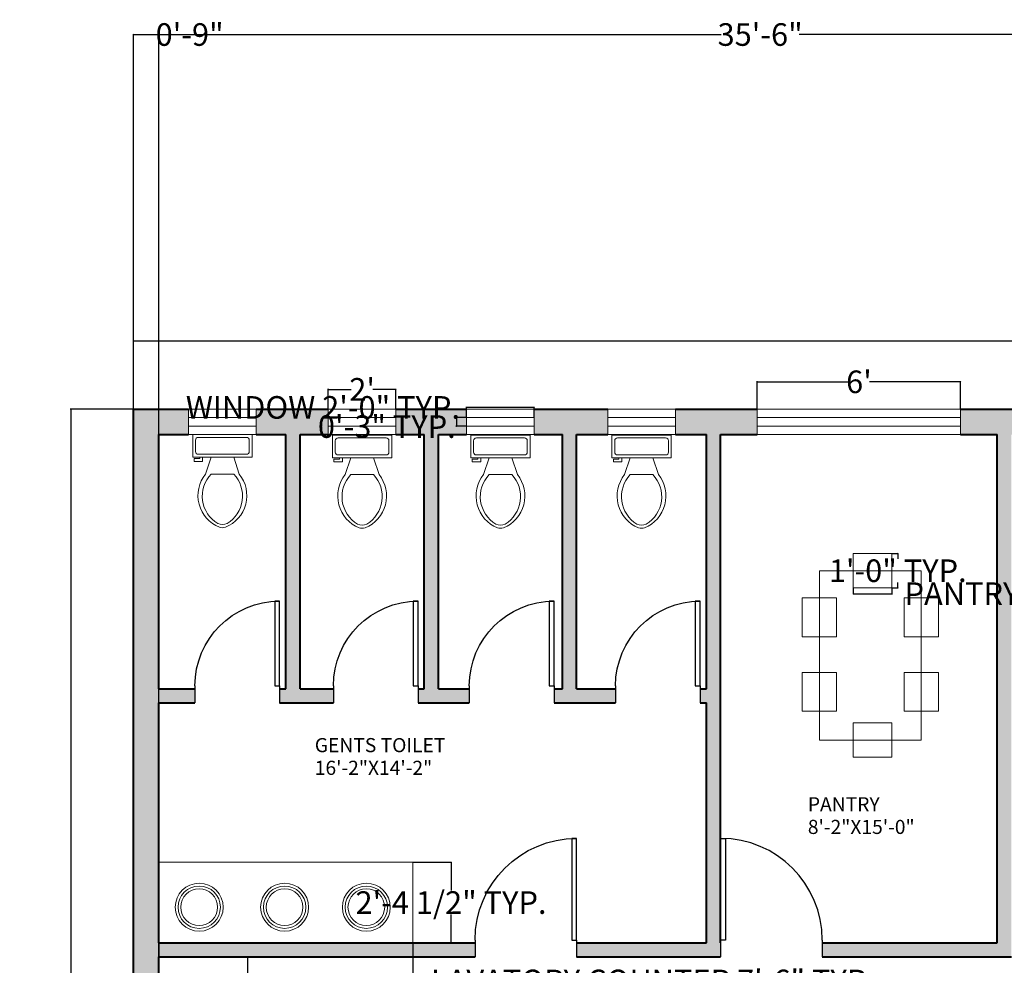
# Model space of a CAD drawing. Units: inches. Extents: x -405 to 940, y 226 to 2032.
# Tile 6 of 10: x -298 to 51, y 1691 to 2026. Entities that reach past the tile are written whole.
import ezdxf

# ---------------------------------------------------------------- set-up
doc = ezdxf.new("R2010")
doc.units = ezdxf.units.IN
doc.header["$MEASUREMENT"] = 0
doc.linetypes.add('ACAD_ISO02W100', pattern=[15, 12, -3])
for name, color, linetype, lineweight in [('A-ANNO-DIMS', 120, 'Continuous', 18), ('A-AREA-IDEN', 32, 'Continuous', 18), ('A-FLOR-FIXT', 175, 'Continuous', 18), ('A-FURN-SEAT', 5, 'Continuous', 18), ('A-GLAZ-HIDN', 1, 'ACAD_ISO02W100', 18), ('A-WALL-PATT', 8, 'Continuous', 13), ('door', 6, 'Continuous', 25), ('tables', 2, 'Continuous', 18), ('wall', 3, 'Continuous', 40), ('window', 1, 'Continuous', 18)]:
    doc.layers.add(name, color=color, linetype=linetype, lineweight=lineweight)
doc.styles.get("Standard").update_dxf_attribs({"font": 'arial.ttf'})
doc.dimstyles.get("Standard").update_dxf_attribs({"dimtxt": 8, "dimasz": 0.18, "dimexe": 0.18, "dimexo": 0.0625, "dimgap": 0.09, "dimtad": 0, "dimtih": 1, "dimtoh": 1, "dimdec": 0, "dimzin": 0, "dimdsep": 46, "dimlunit": 3, "dimtxsty": 'Standard', "dimblk": 'OBLIQUE', "dimcen": 0.09, "dimadec": 0, "dimazin": 0, "dimtfac": 1, "dimtdec": 0, "dimtofl": 0, "dimtmove": 0, "dimatfit": 3, "dimfxl": 1, "dimtolj": 1, "dimtzin": 0, "dimarcsym": 0})

# ---------------------------------------------------------------- blocks, each defined once
blk = doc.blocks.new('*U3')
for p, q in [((0, 0), (0, -6)), ((30, 0), (30, -6))]:
    blk.add_line(p, q)
blk.add_lwpolyline([(0, 0), (0, 30), (1.75, 30), (1.75, 0)], close=True)
blk.add_arc((0, 0), 30, 0, 90)
blk = doc.blocks.new('*U4')
for p, q in [((0, 0), (0, -6)), ((36, 0), (36, -6))]:
    blk.add_line(p, q)
blk.add_lwpolyline([(0, 0), (0, 36), (1.75, 36), (1.75, 0)], close=True)
blk.add_arc((0, 0), 36, 0, 90)
blk = doc.blocks.new('*U6')
for p, q in [((9.5, -6), (9.5, -2)), ((-10, -8.5), (-8, -8.5)), ((-10, -9.5), (-10, -8.5)), ((-7, -9.5), (-10, -9.5)), ((-8, -8.5), (-8, -8)), ((-7, -8), (-7, -9.5)), ((-4, -8), (-6, -14)), ((4, -8), (6, -14)), ((4, -14), (-4, -14))]:
    blk.add_line(p, q)
blk.add_lwpolyline([(10.5, -8), (10.5, 0), (-10.5, 0), (-10.5, -8)], close=True)
for points in [[(-9.5, -2), (-9.5, -6)], [(8.5, -1), (-8.5, -1)], [(-8.5, -7), (8.5, -7)]]:
    blk.add_lwpolyline(points)
for centre, radius, start, end in [((-8.62, -1.88), 0.884, 81.8699, 188.1301), ((8.62, -1.88), 0.884, 351.8699, 98.1301), ((-8.62, -6.12), 0.884, 171.8699, 278.1301), ((8.62, -6.12), 0.884, 261.8699, 8.1301), ((3.52, -21.58), 12.17, 141.4691, 247.9714), ((4.2, -21.82), 11.33, 136.3677, 238.9468), ((-3.52, -21.58), 12.17, 292.0284, 38.5307), ((-4.2, -21.82), 11.33, 301.053, 43.6321), ((0, -27.88), 4, 245.7318, 294.2682), ((0, -29), 4, 254.8605, 285.1395)]:
    blk.add_arc(centre, radius, start, end)
blk = doc.blocks.new('_Oblique')
at = {"color": 0, "linetype": 'ByBlock', "lineweight": -2}
blk.add_line((-0.5, -0.5), (0.5, 0.5), dxfattribs=at)
blk = doc.blocks.new('*D43')
at = {"layer": 'A-ANNO-DIMS', "color": 0, "lineweight": -2, "transparency": 16777216}
for p, q in [((-257.23, 1887.87), (-257.23, 1912.15)), ((-257.23, 1911.97), (265.43, 1911.97)), ((815.77, 1911.97), (293.1, 1911.97)), ((815.77, 1887.87), (815.77, 1912.15))]:
    blk.add_line(p, q, dxfattribs=at)
at = {"layer": 'Defpoints', "color": 0, "transparency": 16777216}
for p in [(815.77, 1911.97), (-257.23, 1887.81), (815.77, 1887.81)]:
    blk.add_point(p, dxfattribs=at)
at = {"layer": 'A-ANNO-DIMS', "color": 0, "lineweight": -2, "transparency": 16777216, "xscale": 0.18, "yscale": 0.18, "zscale": 0.18, "rotation": 180}
blk.add_blockref('_Oblique', (-257.23, 1911.97), dxfattribs=at)
at = {"layer": 'A-ANNO-DIMS', "color": 0, "lineweight": -2, "transparency": 16777216, "xscale": 0.18, "yscale": 0.18, "zscale": 0.18}
blk.add_blockref('_Oblique', (815.77, 1911.97), dxfattribs=at)
at = {"layer": 'A-ANNO-DIMS', "color": 0, "transparency": 16777216, "insert": (279.27, 1911.97), "char_height": 8, "attachment_point": 5}
blk.add_mtext('\\A1;89\'-5"', dxfattribs=at)
blk = doc.blocks.new('*D44')
at = {"layer": 'A-ANNO-DIMS', "color": 0, "lineweight": -2, "transparency": 16777216}
for p, q in [((-257.29, 1887.81), (-279.61, 1887.81)), ((-279.43, 1887.81), (-279.43, 1210.99)), ((-279.43, 525.81), (-279.43, 1202.63)), ((-257.29, 525.81), (-279.61, 525.81))]:
    blk.add_line(p, q, dxfattribs=at)
at = {"layer": 'Defpoints', "color": 0, "transparency": 16777216}
for p in [(-257.23, 1887.81), (-279.43, 525.81), (-257.23, 525.81)]:
    blk.add_point(p, dxfattribs=at)
at = {"layer": 'A-ANNO-DIMS', "color": 0, "lineweight": -2, "transparency": 16777216, "xscale": 0.18, "yscale": 0.18, "zscale": 0.18}
for p, rotation in [((-279.43, 1887.81), 90), ((-279.43, 525.81), 270)]:
    blk.add_blockref('_Oblique', p, dxfattribs=dict(at, rotation=rotation))
at = {"layer": 'A-ANNO-DIMS', "color": 0, "transparency": 16777216, "insert": (-279.43, 1206.81), "char_height": 8, "attachment_point": 5}
blk.add_mtext('\\A1;113\'-6"', dxfattribs=at)
blk = doc.blocks.new('*D59')
at = {"layer": 'A-ANNO-DIMS', "color": 0, "lineweight": -2, "transparency": 16777216}
for p, q in [((-218.67, 1693.81), (-216.61, 1693.81)), ((-216.79, 1693.81), (-216.79, 1655.9)), ((-216.79, 1609.81), (-216.79, 1647.72)), ((-218.67, 1609.81), (-216.61, 1609.81))]:
    blk.add_line(p, q, dxfattribs=at)
at = {"layer": 'Defpoints', "color": 0, "transparency": 16777216}
for p in [(-218.73, 1693.81), (-218.73, 1609.81), (-216.79, 1609.81)]:
    blk.add_point(p, dxfattribs=at)
at = {"layer": 'A-ANNO-DIMS', "color": 0, "lineweight": -2, "transparency": 16777216, "xscale": 0.18, "yscale": 0.18, "zscale": 0.18}
for p, rotation in [((-216.79, 1693.81), 90), ((-216.79, 1609.81), 270)]:
    blk.add_blockref('_Oblique', p, dxfattribs=dict(at, rotation=rotation))
at = {"layer": 'A-ANNO-DIMS', "color": 0, "transparency": 16777216, "insert": (-216.79, 1651.81), "char_height": 8, "attachment_point": 5}
blk.add_mtext("\\A1;7'", dxfattribs=at)
blk = doc.blocks.new('*D61')
at = {"layer": 'A-ANNO-DIMS', "color": 0, "lineweight": -2, "transparency": 16777216}
for p, q in [((-188.23, 1887.87), (-188.23, 1894.99)), ((-188.23, 1894.81), (-180.07, 1894.81)), ((-164.23, 1894.81), (-172.39, 1894.81)), ((-164.23, 1887.87), (-164.23, 1894.99))]:
    blk.add_line(p, q, dxfattribs=at)
at = {"layer": 'Defpoints', "color": 0, "transparency": 16777216}
for p in [(-164.23, 1894.81), (-188.23, 1887.81), (-164.23, 1887.81)]:
    blk.add_point(p, dxfattribs=at)
at = {"layer": 'A-ANNO-DIMS', "color": 0, "lineweight": -2, "transparency": 16777216, "xscale": 0.18, "yscale": 0.18, "zscale": 0.18, "rotation": 180}
blk.add_blockref('_Oblique', (-188.23, 1894.81), dxfattribs=at)
at = {"layer": 'A-ANNO-DIMS', "color": 0, "lineweight": -2, "transparency": 16777216, "xscale": 0.18, "yscale": 0.18, "zscale": 0.18}
blk.add_blockref('_Oblique', (-164.23, 1894.81), dxfattribs=at)
at = {"layer": 'A-ANNO-DIMS', "color": 0, "transparency": 16777216, "insert": (-176.23, 1894.81), "char_height": 8, "attachment_point": 5}
blk.add_mtext("\\A1;2'", dxfattribs=at)
blk = doc.blocks.new('*D62')
at = {"layer": 'A-ANNO-DIMS', "color": 0, "lineweight": -2, "transparency": 16777216}
for p, q in [((-36.23, 1887.87), (-36.23, 1897.66)), ((35.77, 1887.87), (35.77, 1897.66)), ((-36.23, 1897.48), (-4.02, 1897.48)), ((35.77, 1897.48), (3.56, 1897.48))]:
    blk.add_line(p, q, dxfattribs=at)
at = {"layer": 'Defpoints', "color": 0, "transparency": 16777216}
for p in [(35.77, 1897.48), (-36.23, 1887.81), (35.77, 1887.81)]:
    blk.add_point(p, dxfattribs=at)
at = {"layer": 'A-ANNO-DIMS', "color": 0, "lineweight": -2, "transparency": 16777216, "xscale": 0.18, "yscale": 0.18, "zscale": 0.18, "rotation": 180}
blk.add_blockref('_Oblique', (-36.23, 1897.48), dxfattribs=at)
at = {"layer": 'A-ANNO-DIMS', "color": 0, "lineweight": -2, "transparency": 16777216, "xscale": 0.18, "yscale": 0.18, "zscale": 0.18}
blk.add_blockref('_Oblique', (35.77, 1897.48), dxfattribs=at)
at = {"layer": 'A-ANNO-DIMS', "color": 0, "transparency": 16777216, "insert": (-0.23, 1897.48), "char_height": 8, "attachment_point": 5}
blk.add_mtext("\\A1;6'", dxfattribs=at)
blk = doc.blocks.new('LAVATORY-COUNTER-TRIPLE')
for p, q in [((0, 28.51), (89.99, 28.51)), ((89.99, 28.51), (89.99, 0))]:
    blk.add_line(p, q)
for centre, radius in [((14.28, 12.62), 8.5), ((44.55, 12.62), 8.5), ((73.49, 12.62), 8.5), ((14.28, 12.62), 7.5), ((14.28, 12.62), 6.5), ((44.55, 12.62), 7.5), ((44.55, 12.62), 6.5), ((73.49, 12.62), 7.5), ((73.49, 12.62), 6.5)]:
    blk.add_circle(centre, radius)
blk = doc.blocks.new('CHAIR-PANTRY')
blk.add_lwpolyline([(0, 12.15), (13.72, 12.15), (13.72, 0), (0, 0)], close=True)
blk = doc.blocks.new('WIN-PANE-24IN')
for p, q in [((0, 3), (24, 3)), ((0, 0), (24, 0))]:
    blk.add_line(p, q)
blk = doc.blocks.new('WIN-PANE-72IN')
for p, q in [((0, 3), (72, 3)), ((0, 0), (72, 0))]:
    blk.add_line(p, q)
blk = doc.blocks.new('*D85')
at = {"layer": 'A-ANNO-DIMS', "color": 0, "lineweight": -2, "transparency": 16777216}
for p, q in [((-139.23, 1888.41), (-139.41, 1888.41)), ((-139.23, 1884.87), (-139.23, 1888.59)), ((-115.23, 1888.41), (-139.23, 1888.41)), ((-115.23, 1884.87), (-115.23, 1888.59))]:
    blk.add_line(p, q, dxfattribs=at)
at = {"layer": 'Defpoints', "color": 0, "transparency": 16777216}
for p in [(-139.23, 1888.41), (-139.23, 1884.81), (-115.23, 1884.81)]:
    blk.add_point(p, dxfattribs=at)
at = {"layer": 'A-ANNO-DIMS', "color": 0, "lineweight": -2, "transparency": 16777216, "xscale": 0.18, "yscale": 0.18, "zscale": 0.18, "rotation": 180}
blk.add_blockref('_Oblique', (-139.23, 1888.41), dxfattribs=at)
at = {"layer": 'A-ANNO-DIMS', "color": 0, "lineweight": -2, "transparency": 16777216, "xscale": 0.18, "yscale": 0.18, "zscale": 0.18}
blk.add_blockref('_Oblique', (-115.23, 1888.41), dxfattribs=at)
at = {"layer": 'A-ANNO-DIMS', "color": 0, "transparency": 16777216, "insert": (-190.12, 1888.41), "char_height": 8, "attachment_point": 5}
blk.add_mtext('\\A1;WINDOW 2\'-0" TYP.', dxfattribs=at)
blk = doc.blocks.new('*D86')
at = {"layer": 'A-ANNO-DIMS', "color": 0, "lineweight": -2, "transparency": 16777216}
for p, q in [((-139.29, 1884.81), (-143.01, 1884.81)), ((-142.83, 1884.81), (-142.83, 1881.81)), ((-139.29, 1881.81), (-143.01, 1881.81)), ((-142.83, 1881.63), (-143.01, 1881.63)), ((-142.83, 1881.81), (-142.83, 1881.63))]:
    blk.add_line(p, q, dxfattribs=at)
at = {"layer": 'Defpoints', "color": 0, "transparency": 16777216}
for p in [(-139.23, 1884.81), (-142.83, 1881.81), (-139.23, 1881.81)]:
    blk.add_point(p, dxfattribs=at)
at = {"layer": 'A-ANNO-DIMS', "color": 0, "lineweight": -2, "transparency": 16777216, "xscale": 0.18, "yscale": 0.18, "zscale": 0.18}
for p, rotation in [((-142.83, 1884.81), 90), ((-142.83, 1881.81), 270)]:
    blk.add_blockref('_Oblique', p, dxfattribs=dict(at, rotation=rotation))
at = {"layer": 'A-ANNO-DIMS', "color": 0, "transparency": 16777216, "insert": (-167.48, 1881.63), "char_height": 8, "attachment_point": 5}
blk.add_mtext('\\A1;0\'-3" TYP.', dxfattribs=at)
blk = doc.blocks.new('*D91')
at = {"layer": 'A-ANNO-DIMS', "color": 0, "lineweight": -2, "transparency": 16777216}
for p, q in [((-2.26, 1824.45), (-2.26, 1822.27)), ((11.46, 1824.45), (11.46, 1822.27)), ((-2.26, 1822.45), (11.46, 1822.45)), ((11.46, 1822.45), (11.64, 1822.45))]:
    blk.add_line(p, q, dxfattribs=at)
at = {"layer": 'Defpoints', "color": 0, "transparency": 16777216}
for p in [(-2.26, 1824.51), (11.46, 1824.51), (11.46, 1822.45)]:
    blk.add_point(p, dxfattribs=at)
at = {"layer": 'A-ANNO-DIMS', "color": 0, "lineweight": -2, "transparency": 16777216, "xscale": 0.18, "yscale": 0.18, "zscale": 0.18, "rotation": 180}
blk.add_blockref('_Oblique', (-2.26, 1822.45), dxfattribs=at)
at = {"layer": 'A-ANNO-DIMS', "color": 0, "lineweight": -2, "transparency": 16777216, "xscale": 0.18, "yscale": 0.18, "zscale": 0.18}
blk.add_blockref('_Oblique', (11.46, 1822.45), dxfattribs=at)
at = {"layer": 'A-ANNO-DIMS', "color": 0, "transparency": 16777216, "insert": (88.39, 1822.45), "char_height": 8, "attachment_point": 5}
blk.add_mtext('\\A1;PANTRY CHAIR 1\'-1 1/2" TYP.', dxfattribs=at)
blk = doc.blocks.new('*D92')
at = {"layer": 'A-ANNO-DIMS', "color": 0, "lineweight": -2, "transparency": 16777216}
for p, q in [((11.53, 1836.66), (13.7, 1836.66)), ((13.52, 1836.66), (13.52, 1834.76)), ((11.53, 1824.51), (13.7, 1824.51)), ((13.52, 1824.51), (13.52, 1826.41))]:
    blk.add_line(p, q, dxfattribs=at)
at = {"layer": 'Defpoints', "color": 0, "transparency": 16777216}
for p in [(11.46, 1836.66), (13.52, 1836.66), (11.46, 1824.51)]:
    blk.add_point(p, dxfattribs=at)
at = {"layer": 'A-ANNO-DIMS', "color": 0, "lineweight": -2, "transparency": 16777216, "xscale": 0.18, "yscale": 0.18, "zscale": 0.18}
for p, rotation in [((13.52, 1836.66), 90), ((13.52, 1824.51), 270)]:
    blk.add_blockref('_Oblique', p, dxfattribs=dict(at, rotation=rotation))
at = {"layer": 'A-ANNO-DIMS', "color": 0, "transparency": 16777216, "insert": (13.52, 1830.58), "char_height": 8, "attachment_point": 5}
blk.add_mtext('\\A1;1\'-0" TYP.', dxfattribs=at)
blk = doc.blocks.new('*D93')
at = {"layer": 'A-ANNO-DIMS', "color": 0, "lineweight": -2, "transparency": 16777216}
for p, q in [((-248.23, 1698.75), (-248.23, 1685.13)), ((-158.24, 1698.75), (-158.24, 1685.13)), ((-248.23, 1685.31), (-158.24, 1685.31)), ((-158.24, 1685.31), (-158.06, 1685.31))]:
    blk.add_line(p, q, dxfattribs=at)
at = {"layer": 'Defpoints', "color": 0, "transparency": 16777216}
for p in [(-248.23, 1698.81), (-158.24, 1698.81), (-158.24, 1685.31)]:
    blk.add_point(p, dxfattribs=at)
at = {"layer": 'A-ANNO-DIMS', "color": 0, "lineweight": -2, "transparency": 16777216, "xscale": 0.18, "yscale": 0.18, "zscale": 0.18, "rotation": 180}
blk.add_blockref('_Oblique', (-248.23, 1685.31), dxfattribs=at)
at = {"layer": 'A-ANNO-DIMS', "color": 0, "lineweight": -2, "transparency": 16777216, "xscale": 0.18, "yscale": 0.18, "zscale": 0.18}
blk.add_blockref('_Oblique', (-158.24, 1685.31), dxfattribs=at)
at = {"layer": 'A-ANNO-DIMS', "color": 0, "transparency": 16777216, "insert": (-73.22, 1685.31), "char_height": 8, "attachment_point": 5}
blk.add_mtext('\\A1;LAVATORY COUNTER 7\'-6" TYP.', dxfattribs=at)
blk = doc.blocks.new('*D94')
at = {"layer": 'A-ANNO-DIMS', "color": 0, "lineweight": -2, "transparency": 16777216}
for p, q in [((-158.18, 1727.32), (-144.56, 1727.32)), ((-144.74, 1727.32), (-144.74, 1717.29)), ((-144.74, 1698.81), (-144.74, 1708.84)), ((-158.18, 1698.81), (-144.56, 1698.81))]:
    blk.add_line(p, q, dxfattribs=at)
at = {"layer": 'Defpoints', "color": 0, "transparency": 16777216}
for p in [(-158.24, 1727.32), (-144.74, 1727.32), (-158.24, 1698.81)]:
    blk.add_point(p, dxfattribs=at)
at = {"layer": 'A-ANNO-DIMS', "color": 0, "lineweight": -2, "transparency": 16777216, "xscale": 0.18, "yscale": 0.18, "zscale": 0.18}
for p, rotation in [((-144.74, 1727.32), 90), ((-144.74, 1698.81), 270)]:
    blk.add_blockref('_Oblique', p, dxfattribs=dict(at, rotation=rotation))
at = {"layer": 'A-ANNO-DIMS', "color": 0, "transparency": 16777216, "insert": (-144.74, 1713.07), "char_height": 8, "attachment_point": 5}
blk.add_mtext('\\A1;2\'-4 1/2" TYP.', dxfattribs=at)
blk = doc.blocks.new('*D109')
at = {"layer": 'A-ANNO-DIMS', "color": 0, "lineweight": -2, "transparency": 16777216}
for p, q in [((-248.23, 750.87), (-248.23, 2020.64)), ((-248.23, 2020.46), (-49.06, 2020.46)), ((177.77, 2020.46), (-21.4, 2020.46)), ((177.77, 750.87), (177.77, 2020.64))]:
    blk.add_line(p, q, dxfattribs=at)
at = {"layer": 'Defpoints', "color": 0, "transparency": 16777216}
for p in [(177.77, 2020.46), (-248.23, 750.81), (177.77, 750.81)]:
    blk.add_point(p, dxfattribs=at)
at = {"layer": 'A-ANNO-DIMS', "color": 0, "lineweight": -2, "transparency": 16777216, "xscale": 0.18, "yscale": 0.18, "zscale": 0.18, "rotation": 180}
blk.add_blockref('_Oblique', (-248.23, 2020.46), dxfattribs=at)
at = {"layer": 'A-ANNO-DIMS', "color": 0, "lineweight": -2, "transparency": 16777216, "xscale": 0.18, "yscale": 0.18, "zscale": 0.18}
blk.add_blockref('_Oblique', (177.77, 2020.46), dxfattribs=at)
at = {"layer": 'A-ANNO-DIMS', "color": 0, "transparency": 16777216, "insert": (-35.23, 2020.46), "char_height": 8, "attachment_point": 5}
blk.add_mtext('\\A1;35\'-6"', dxfattribs=at)
blk = doc.blocks.new('*D115')
at = {"layer": 'A-ANNO-DIMS', "color": 0, "lineweight": -2, "transparency": 16777216}
for p, q in [((-257.23, 1887.87), (-257.23, 2020.64)), ((-257.23, 2020.46), (-248.23, 2020.46)), ((-248.23, 1878.87), (-248.23, 2020.64)), ((-248.23, 2020.46), (-248.05, 2020.46))]:
    blk.add_line(p, q, dxfattribs=at)
at = {"layer": 'Defpoints', "color": 0, "transparency": 16777216}
for p in [(-248.23, 2020.46), (-257.23, 1887.81), (-248.23, 1878.81)]:
    blk.add_point(p, dxfattribs=at)
at = {"layer": 'A-ANNO-DIMS', "color": 0, "lineweight": -2, "transparency": 16777216, "xscale": 0.18, "yscale": 0.18, "zscale": 0.18, "rotation": 180}
blk.add_blockref('_Oblique', (-257.23, 2020.46), dxfattribs=at)
at = {"layer": 'A-ANNO-DIMS', "color": 0, "lineweight": -2, "transparency": 16777216, "xscale": 0.18, "yscale": 0.18, "zscale": 0.18}
blk.add_blockref('_Oblique', (-248.23, 2020.46), dxfattribs=at)
at = {"layer": 'A-ANNO-DIMS', "color": 0, "transparency": 16777216, "insert": (-237.33, 2020.46), "char_height": 8, "attachment_point": 5}
blk.add_mtext('\\A1;0\'-9"', dxfattribs=at)

msp = doc.modelspace()

# ---------------------------------------------------------------- hatches: boundary and pattern name
at = {"layer": 'A-WALL-PATT'}
h = msp.add_hatch(dxfattribs=at)
h.set_pattern_fill('AR-HBONE', color=256)
h.set_pattern_definition([(45, (599.8442, 904.9158), (0, 5.656854), [12, -4]), (135, (602.6726, 907.744), (4e-16, 5.656854), [12, -4])])
h.paths.add_polyline_path([(-248.23, 1045.81), (-257.23, 1045.81), (-257.23, 964.81), (-248.23, 964.81)], flags=17)
h.paths.add_polyline_path([(-248.23, 851.81), (-39.23, 851.81), (-39.23, 856.81), (-44.23, 856.81), (-248.23, 856.81), (-248.23, 892.81), (-257.23, 892.81), (-257.23, 839.81), (-248.23, 839.81)])
h.paths.add_polyline_path([(-248.23, 750.81), (124.74, 750.81), (124.74, 751.73), (124.74, 755.81), (-248.23, 755.81), (-248.23, 767.81), (-257.23, 767.81), (-257.23, 726.81), (-248.23, 726.81)])
h.paths.add_polyline_path([(-248.23, 654.81), (-257.23, 654.81), (-257.23, 630.81), (-248.23, 630.81)])
h.paths.add_polyline_path([(-180.23, 534.81), (-248.23, 534.81), (-248.23, 558.81), (-257.23, 558.81), (-257.23, 525.81), (-180.23, 525.81)])
h.paths.add_polyline_path([(-69.23, 534.81), (-108.23, 534.81), (-108.23, 525.81), (-69.23, 525.81)])
h.paths.add_polyline_path([(35.77, 534.81), (2.77, 534.81), (2.77, 525.81), (35.77, 525.81)])
h.paths.add_polyline_path([(182.77, 755.81), (160.74, 755.81), (160.74, 750.81), (177.77, 750.81), (177.77, 534.81), (107.77, 534.81), (107.77, 525.81), (182.77, 525.81)])
h.paths.add_polyline_path([(-39.23, 1609.81), (-44.23, 1609.81), (-44.23, 1604.81), (-44.23, 1460.81), (-135.23, 1460.81), (-135.23, 1465.73), (-140.23, 1465.73), (-140.23, 1460.81), (-248.23, 1460.81), (-248.23, 1471.31), (-257.23, 1471.31), (-257.23, 1419.81), (-248.23, 1419.81), (-248.23, 1455.81), (-44.23, 1455.81), (-44.23, 1194.81), (-39.23, 1194.81)])
h.paths.add_polyline_path([(-248.23, 1520.81), (-257.23, 1520.81), (-257.23, 1495.31), (-248.23, 1495.31), (-248.23, 1505.81), (-140.23, 1505.81), (-140.23, 1495.73), (-135.23, 1495.73), (-135.23, 1516.79), (-140.23, 1516.79), (-140.23, 1510.81), (-248.23, 1510.81)], flags=17)
h.paths.add_polyline_path([(-248.23, 1570.31), (-257.23, 1570.31), (-257.23, 1544.81), (-248.23, 1544.81), (-248.23, 1554.81), (-140.23, 1554.81), (-140.23, 1546.79), (-135.23, 1546.79), (-135.23, 1565.08), (-140.23, 1565.08), (-140.23, 1559.81), (-248.23, 1559.81)], flags=17)
h.paths.add_polyline_path([(-248.23, 1615.81), (-257.23, 1615.81), (-257.23, 1594.31), (-248.23, 1594.31), (-248.23, 1604.81), (-140.23, 1604.81), (-140.23, 1595.08), (-135.23, 1595.08), (-135.23, 1604.81), (-80.23, 1604.81), (-80.23, 1609.81), (-248.23, 1609.81)])
h.paths.add_polyline_path([(-248.23, 1783.81), (-235.46, 1783.81), (-235.46, 1788.81), (-248.23, 1788.81), (-248.23, 1878.81), (-237.73, 1878.81), (-237.73, 1887.81), (-257.23, 1887.81), (-257.23, 1687.81), (-248.23, 1687.81), (-248.23, 1693.81), (-136.23, 1693.81), (-136.23, 1698.81), (-248.23, 1698.81)])
h.paths.add_polyline_path([(-188.23, 1887.81), (-213.73, 1887.81), (-213.73, 1878.81), (-203.23, 1878.81), (-203.23, 1788.81), (-205.46, 1788.81), (-205.46, 1783.81), (-186.39, 1783.81), (-186.39, 1788.81), (-198.23, 1788.81), (-198.23, 1878.81), (-188.23, 1878.81)])
h.paths.add_polyline_path([(-139.23, 1887.81), (-164.23, 1887.81), (-164.23, 1878.81), (-154.23, 1878.81), (-154.23, 1788.81), (-156.39, 1788.81), (-156.39, 1783.81), (-138.25, 1783.81), (-138.25, 1788.81), (-149.23, 1788.81), (-149.23, 1878.81), (-139.23, 1878.81)])
h.paths.add_polyline_path([(-89.23, 1887.81), (-115.23, 1887.81), (-115.23, 1878.81), (-105.23, 1878.81), (-105.23, 1788.81), (-108.25, 1788.81), (-108.25, 1783.81), (-86.45, 1783.81), (-86.45, 1788.81), (-100.23, 1788.81), (-100.23, 1878.81), (-89.23, 1878.81)])
h.paths.add_polyline_path([(-36.23, 1887.81), (-65.23, 1887.81), (-65.23, 1878.81), (-54.23, 1878.81), (-54.23, 1788.81), (-56.45, 1788.81), (-56.45, 1783.81), (-54.23, 1783.81), (-54.23, 1698.81), (-100.23, 1698.81), (-100.23, 1693.81), (-49.23, 1693.81), (-49.23, 1698.81), (-49.23, 1878.81), (-36.23, 1878.81)])
h.paths.add_polyline_path([(89.77, 1887.81), (35.77, 1887.81), (35.77, 1878.81), (48.77, 1878.81), (48.77, 1698.81), (-13.23, 1698.81), (-13.23, 1693.81), (53.77, 1693.81), (53.77, 1698.81), (53.77, 1878.81), (89.77, 1878.81)])
h.paths.add_polyline_path([(255.27, 1887.81), (161.77, 1887.81), (161.77, 1878.81), (197.77, 1878.81), (197.77, 1698.81), (89.77, 1698.81), (89.77, 1693.81), (202.77, 1693.81), (202.77, 1698.81), (202.77, 1878.81), (255.27, 1878.81)])
h.paths.add_polyline_path([(375.27, 1887.81), (327.27, 1887.81), (327.27, 1878.81), (375.27, 1878.81)], flags=17)
h.paths.add_polyline_path([(815.77, 1887.81), (447.27, 1887.81), (447.27, 1878.81), (499.77, 1878.81), (499.77, 1698.81), (238.77, 1698.81), (238.77, 1693.81), (504.77, 1693.81), (504.77, 1878.81), (633.77, 1878.81), (633.77, 1646.81), (597.77, 1646.81), (597.77, 1641.81), (602.77, 1641.81), (638.77, 1641.81), (638.77, 1878.81), (806.77, 1878.81), (806.77, 1838.31), (815.77, 1838.31)])
h.paths.add_polyline_path([(815.77, 1766.31), (806.77, 1766.31), (806.77, 1718.31), (815.77, 1718.31)], flags=17)
h.paths.add_polyline_path([(815.77, 1356.31), (806.77, 1356.31), (806.77, 1303.81), (602.77, 1303.81), (597.77, 1303.81), (597.77, 1037.81), (602.77, 1037.81), (602.77, 1298.81), (806.77, 1298.81), (806.77, 1246.31), (815.77, 1246.31)])
h.paths.add_polyline_path([(815.77, 1174.31), (806.77, 1174.31), (806.77, 1126.31), (815.77, 1126.31)], flags=17)
h.paths.add_polyline_path([(815.77, 1054.31), (806.77, 1054.31), (806.77, 1001.81), (796.08, 1001.81), (796.08, 1001.75), (780.86, 1001.75), (602.77, 1001.81), (597.77, 1001.81), (597.77, 892.81), (602.77, 892.81), (602.77, 996.81), (806.77, 996.81), (806.77, 962.81), (815.77, 962.81)])
h.paths.add_polyline_path([(403.77, 534.81), (379.77, 534.81), (379.77, 525.81), (403.77, 525.81)])
h.paths.add_polyline_path([(-39.23, 1158.81), (-44.23, 1158.81), (-248.23, 1158.81), (-248.23, 1194.81), (-257.23, 1194.81), (-257.23, 1117.81), (-248.23, 1117.81), (-248.23, 1153.81), (-44.23, 1153.81), (-44.23, 892.81), (-39.23, 892.81)])
h.paths.add_polyline_path([(-248.23, 1347.81), (-257.23, 1347.81), (-257.23, 1275.81), (-248.23, 1275.81)], flags=17)
h.paths.add_polyline_path([(815.77, 1476.31), (806.77, 1476.31), (806.77, 1428.31), (815.77, 1428.31)], flags=17)
h.paths.add_polyline_path([(815.77, 1646.31), (806.77, 1646.31), (806.77, 1638.65), (806.77, 1605.81), (597.77, 1605.81), (597.77, 1339.81), (602.77, 1339.81), (602.77, 1600.81), (806.77, 1600.81), (806.77, 1548.31), (815.77, 1548.31)])

# ---------------------------------------------------------------- linework, layer by layer
at = {"layer": 'A-GLAZ-HIDN'}
for p, q in [((-237.73, 1878.81), (-237.73, 1887.81)), ((-213.73, 1878.81), (-213.73, 1887.81)), ((-188.23, 1878.81), (-188.23, 1887.81)), ((-164.23, 1878.81), (-164.23, 1887.81)), ((-139.23, 1878.81), (-139.23, 1887.81)), ((-115.23, 1878.81), (-115.23, 1887.81)), ((-89.23, 1878.81), (-89.23, 1887.81)), ((-65.23, 1878.81), (-65.23, 1887.81)), ((-36.23, 1878.81), (-36.23, 1887.81)), ((35.77, 1878.81), (35.77, 1887.81))]:
    msp.add_line(p, q, dxfattribs=at)
at = {"layer": 'door'}
for p, q in [((-235.46, 1788.81), (-235.46, 1783.81)), ((-205.46, 1788.81), (-205.46, 1783.81)), ((-186.39, 1788.81), (-186.39, 1783.81)), ((-156.39, 1788.81), (-156.39, 1783.81)), ((-138.25, 1788.81), (-138.25, 1783.81)), ((-108.25, 1788.81), (-108.25, 1783.81)), ((-86.45, 1788.81), (-86.45, 1783.81)), ((-56.45, 1788.81), (-56.45, 1783.81)), ((-136.23, 1698.81), (-136.23, 1693.81)), ((-100.23, 1698.81), (-100.23, 1693.81)), ((-49.23, 1698.81), (-49.23, 1693.81)), ((-13.23, 1698.81), (-13.23, 1693.81))]:
    msp.add_line(p, q, dxfattribs=at)
at = {"layer": 'tables'}
msp.add_lwpolyline([(21.83, 1830.58), (-14.17, 1830.58), (-14.17, 1770.58), (21.83, 1770.58)], close=True, dxfattribs=at)
at = {"layer": 'wall'}
for p, q in [((-257.23, 1887.81), (-237.73, 1887.81)), ((-257.23, 1687.81), (-257.23, 1887.81)), ((-213.73, 1887.81), (-188.23, 1887.81)), ((-164.23, 1887.81), (-139.23, 1887.81)), ((-115.23, 1887.81), (-89.23, 1887.81)), ((-65.23, 1887.81), (-36.23, 1887.81)), ((35.77, 1887.81), (89.77, 1887.81)), ((-248.23, 1878.81), (-237.73, 1878.81)), ((-248.23, 1788.81), (-248.23, 1878.81)), ((-213.73, 1878.81), (-203.23, 1878.81)), ((-203.23, 1788.81), (-203.23, 1878.81)), ((-198.23, 1878.81), (-188.23, 1878.81)), ((-198.23, 1788.81), (-198.23, 1878.81)), ((-164.23, 1878.81), (-154.23, 1878.81)), ((-154.23, 1788.81), (-154.23, 1878.81)), ((-149.23, 1788.81), (-149.23, 1878.81)), ((-149.23, 1878.81), (-139.23, 1878.81)), ((-115.23, 1878.81), (-105.23, 1878.81)), ((-105.23, 1788.81), (-105.23, 1878.81)), ((-100.23, 1788.81), (-100.23, 1878.81)), ((-100.23, 1878.81), (-89.23, 1878.81)), ((-65.23, 1878.81), (-54.23, 1878.81)), ((-54.23, 1788.81), (-54.23, 1878.81)), ((-49.23, 1698.81), (-49.23, 1878.81)), ((-49.23, 1878.81), (-36.23, 1878.81)), ((35.77, 1878.81), (48.77, 1878.81)), ((48.77, 1698.81), (48.77, 1878.81)), ((-248.23, 1788.81), (-235.46, 1788.81)), ((-205.46, 1788.81), (-203.23, 1788.81)), ((-198.23, 1788.81), (-186.39, 1788.81)), ((-156.39, 1788.81), (-154.23, 1788.81)), ((-149.23, 1788.81), (-138.25, 1788.81)), ((-108.25, 1788.81), (-105.23, 1788.81)), ((-100.23, 1788.81), (-86.45, 1788.81)), ((-56.45, 1788.81), (-54.23, 1788.81)), ((-248.23, 1698.81), (-248.23, 1783.81)), ((-248.23, 1783.81), (-235.46, 1783.81)), ((-205.46, 1783.81), (-186.39, 1783.81)), ((-156.39, 1783.81), (-138.25, 1783.81)), ((-108.25, 1783.81), (-86.45, 1783.81)), ((-56.45, 1783.81), (-54.23, 1783.81)), ((-54.23, 1698.81), (-54.23, 1783.81)), ((-248.23, 1698.81), (-136.23, 1698.81)), ((-100.23, 1698.81), (-54.23, 1698.81)), ((-13.23, 1698.81), (48.77, 1698.81)), ((-248.23, 1693.81), (-136.23, 1693.81)), ((-248.23, 1687.81), (-248.23, 1693.81)), ((-100.23, 1693.81), (-49.23, 1693.81)), ((-13.23, 1693.81), (53.77, 1693.81))]:
    msp.add_line(p, q, dxfattribs=at)
at = {"layer": 'window'}
for p, q in [((-237.73, 1887.81), (-213.73, 1887.81)), ((-188.23, 1887.81), (-164.23, 1887.81)), ((-139.23, 1887.81), (-115.23, 1887.81)), ((-89.23, 1887.81), (-65.23, 1887.81)), ((-36.23, 1887.81), (35.77, 1887.81)), ((-237.73, 1878.81), (-213.73, 1878.81)), ((-188.23, 1878.81), (-164.23, 1878.81)), ((-139.23, 1878.81), (-115.23, 1878.81)), ((-89.23, 1878.81), (-65.23, 1878.81)), ((-36.23, 1878.81), (35.77, 1878.81))]:
    msp.add_line(p, q, dxfattribs=at)

# ---------------------------------------------------------------- block references
at = {"layer": 'A-FLOR-FIXT'}
for name, p in [('*U6', (-225.73, 1878.81)), ('*U6', (-176.23, 1878.6)), ('*U6', (-127.23, 1878.6)), ('*U6', (-77.23, 1878.6)), ('LAVATORY-COUNTER-TRIPLE', (-248.23, 1698.81))]:
    msp.add_blockref(name, p, dxfattribs=at)
at = {"layer": 'A-FURN-SEAT'}
msp.add_blockref('CHAIR-PANTRY', (-2.26, 1824.51), dxfattribs=at)
for p, rotation in [((-20.35, 1820.95), 270.0000000000017), ((-20.35, 1794.58), 270.0000000000032)]:
    msp.add_blockref('CHAIR-PANTRY', p, dxfattribs=dict(at, rotation=rotation))
at = {"layer": 'A-FURN-SEAT', "extrusion": (0, 0, -1), "zscale": -1}
for p, rotation in [((-28, 1820.95), 270.0000000000017), ((-28, 1794.58), 270.0000000000032), ((2.26, 1776.66), 180)]:
    msp.add_blockref('CHAIR-PANTRY', p, dxfattribs=dict(at, rotation=rotation))
at = {"layer": 'door', "xscale": -1}
for name, p in [('*U3', (-205.46, 1789.81)), ('*U3', (-156.39, 1789.81)), ('*U3', (-108.25, 1789.81)), ('*U3', (-56.45, 1789.81)), ('*U4', (-100.23, 1699.81))]:
    msp.add_blockref(name, p, dxfattribs=at)
at = {"layer": 'door'}
msp.add_blockref('*U4', (-49.23, 1699.81), dxfattribs=at)
at = {"layer": 'window'}
for name, p in [('WIN-PANE-24IN', (-237.73, 1881.81)), ('WIN-PANE-72IN', (-36.23, 1881.81))]:
    msp.add_blockref(name, p, dxfattribs=at)
at = {"layer": 'window', "rotation": 180}
for p in [(-164.23, 1884.81), (-115.23, 1884.81), (-65.23, 1884.81)]:
    msp.add_blockref('WIN-PANE-24IN', p, dxfattribs=at)

# ---------------------------------------------------------------- texts
at = {"layer": 'A-AREA-IDEN'}
for s, p in [('GENTS TOILET ', (-193.01, 1766.32)), ('16\'-2"X14\'-2"', (-193.01, 1758.29)), ('PANTRY ', (-18.33, 1745.39)), ('8\'-2"X15\'-0"', (-18.33, 1737.36))]:
    msp.add_text(s, height=5, dxfattribs=at).set_placement(p)

# ---------------------------------------------------------------- dimensions: what is measured, and where the dimension line sits
at = {"layer": 'A-ANNO-DIMS'}
for base, p1, p2, override, picture, middle in [((-248.23, 2020.46), (-257.23, 1887.81), (-248.23, 1878.81), {"dimdec": 1, "dimlfac": 1, "dimrnd": 0, "dimzin": 1, "dimdsep": 46, "dimlunit": 4, "dimfrac": 2}, '*D115', (-237.33, 2020.46)), ((177.77, 2020.46), (-248.23, 750.81), (177.77, 750.81), {"dimdec": 1, "dimlfac": 1, "dimrnd": 0, "dimzin": 1, "dimdsep": 46, "dimlunit": 4, "dimfrac": 2}, '*D109', (-35.23, 2020.46)), ((815.77, 1911.97), (-257.23, 1887.81), (815.77, 1887.81), {"dimclrd": 0, "dimclre": 0, "dimclrt": 0}, '*D43', (279.27, 1911.97)), ((35.77, 1897.48), (-36.23, 1887.81), (35.77, 1887.81), {"dimclrd": 0, "dimclre": 0, "dimclrt": 0}, '*D62', (-0.23, 1897.48)), ((-164.23, 1894.81), (-188.23, 1887.81), (-164.23, 1887.81), {"dimclrd": 0, "dimclre": 0, "dimclrt": 0}, '*D61', (-176.23, 1894.81))]:
    dim = msp.add_linear_dim(base=base, p1=p1, p2=p2, dimstyle='Standard', override=override, dxfattribs=at)
    dim.commit()
    dim.dimension.update_dxf_attribs({"geometry": picture, "text_midpoint": middle})
for base, p1, p2, angle, text, picture, middle in [((-139.23, 1888.41), (-115.23, 1884.81), (-139.23, 1884.81), 180, 'WINDOW <> TYP.', '*D85', (-190.12, 1888.41)), ((-142.83, 1881.81), (-139.23, 1884.81), (-139.23, 1881.81), 270, '<> TYP.', '*D86', (-167.48, 1881.63)), ((13.5205, 1836.6604), (11.4625, 1824.5088), (11.4625, 1836.6604), 90, '<> TYP.', '*D92', (13.5205, 1830.5846)), ((-144.74, 1727.32), (-158.24, 1698.81), (-158.24, 1727.32), 90, '<> TYP.', '*D94', (-144.74, 1713.07))]:
    dim = msp.add_linear_dim(base=base, p1=p1, p2=p2, angle=angle, text=text, dimstyle='Standard', override={"dimdec": 1, "dimlfac": 1, "dimrnd": 0, "dimzin": 1, "dimdsep": 46, "dimlunit": 4, "dimfrac": 2}, dxfattribs=at)
    dim.commit()
    dim.dimension.update_dxf_attribs({"geometry": picture, "text_midpoint": middle})
for base, p1, p2, picture, middle in [((-279.43, 525.81), (-257.23, 1887.81), (-257.23, 525.81), '*D44', (-279.43, 1206.81)), ((-216.79, 1609.81), (-218.73, 1693.81), (-218.73, 1609.81), '*D59', (-216.79, 1651.81))]:
    dim = msp.add_linear_dim(base=base, p1=p1, p2=p2, angle=90, dimstyle='Standard', override={"dimclrd": 0, "dimclre": 0, "dimclrt": 0}, dxfattribs=at)
    dim.commit()
    dim.dimension.update_dxf_attribs({"geometry": picture, "text_midpoint": middle})
for base, p1, p2, text, picture, middle in [((11.46, 1822.45), (-2.26, 1824.51), (11.46, 1824.51), 'PANTRY CHAIR <> TYP.', '*D91', (88.39, 1822.45)), ((-158.24, 1685.31), (-248.23, 1698.81), (-158.24, 1698.81), 'LAVATORY COUNTER <> TYP.', '*D93', (-73.22, 1685.31))]:
    dim = msp.add_linear_dim(base=base, p1=p1, p2=p2, text=text, dimstyle='Standard', override={"dimdec": 1, "dimlfac": 1, "dimrnd": 0, "dimzin": 1, "dimdsep": 46, "dimlunit": 4, "dimfrac": 2}, dxfattribs=at)
    dim.commit()
    dim.dimension.update_dxf_attribs({"geometry": picture, "text_midpoint": middle})

doc.saveas('drawing.dxf')
